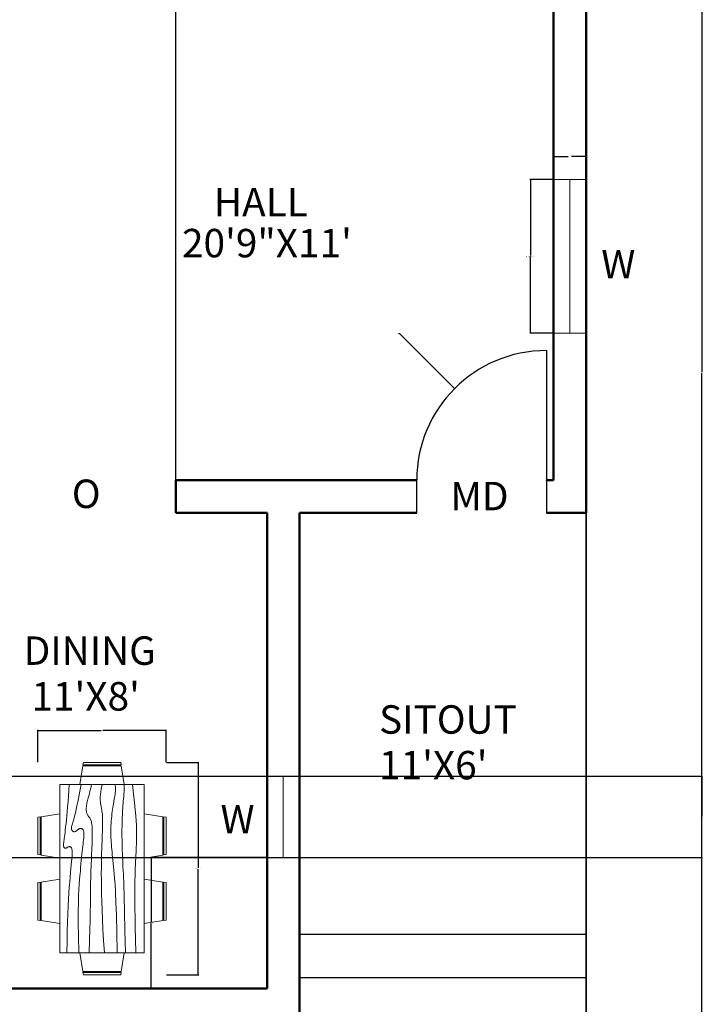
# Model space of a CAD drawing. Units: feet. Extents: x 1657 to 2001, y 1678 to 2367.
# Tile 3 of 4: x 1811 to 2001, y 1847 to 2120. Entities that reach past the tile are written whole.
import ezdxf

# ---------------------------------------------------------------- set-up
doc = ezdxf.new("R2010")
doc.units = ezdxf.units.FT
for name, color, linetype, lineweight in [('A-ANNO-DIMS', 2, 'Continuous', 18), ('A-ANNO-TEXT', 7, 'Continuous', 18), ('A-AREA-IDEN', 7, 'Continuous', 25), ('A-DOOR', 3, 'Continuous', 25), ('A-FLOR', 7, 'Continuous', 35), ('A-FLOR-STRS', 7, 'Continuous', 25), ('A-FURN', 8, 'Continuous', 18), ('A-GLAZ', 4, 'Continuous', 18), ('A-WALL', 7, 'Continuous', 50)]:
    doc.layers.add(name, color=color, linetype=linetype, lineweight=lineweight)
doc.styles.get("Standard").update_dxf_attribs({"font": 'arial.ttf'})
doc.dimstyles.get("Standard").update_dxf_attribs({"dimtxt": 0.18, "dimasz": 0.18, "dimexe": 0.18, "dimexo": 0.0625, "dimgap": 0.09, "dimtad": 0, "dimtih": 1, "dimtoh": 1, "dimdec": 4, "dimzin": 0, "dimdsep": 46, "dimtxsty": 'Standard', "dimcen": 0.09, "dimadec": 0, "dimazin": 0, "dimtfac": 1, "dimtdec": 4, "dimtofl": 0, "dimtmove": 0, "dimatfit": 3, "dimfxl": 1, "dimtolj": 1, "dimtzin": 0, "dimarcsym": 0})

# ---------------------------------------------------------------- blocks, each defined once
blk = doc.blocks.new('Dining Set - 36 x 72 in.')
for p, q in [((-22.2343, 26.00059), (-23.4847, 17.99762)), ((-22.2304, 26), (-5.7608, 26)), ((-22, 27.5), (-22.1562, 26.50042)), ((-5.8416, 26.5), (-22.1534, 26.5)), ((-22, 27.5), (-6, 27.5)), ((-5.8437, 26.49966), (-6, 27.5)), ((-4.5152, 17.99762), (-5.7655, 25.99926)), ((5.7657, 26.00059), (4.5153, 17.99762)), ((5.7696, 26), (22.2392, 26)), ((6, 27.5), (5.8438, 26.50042)), ((22.1584, 26.5), (5.8466, 26.5)), ((6, 27.5), (22, 27.5)), ((22.1563, 26.49966), (22, 27.5)), ((23.4848, 17.99762), (22.2345, 25.99926)), ((36, 18), (-36, 18)), ((-36, 18), (-36, -18)), ((36, -18), (36, 18)), ((-44.0006, 8.23428), (-35.9976, 9.48474)), ((44.0006, 8.23428), (35.9976, 9.48474)), ((-45.5, 8), (-44.5004, 8.15617)), ((-45.5, 8), (-45.5, -8)), ((-44.5, -8.15843), (-44.5, 8.15338)), ((-44, 8.23041), (-44, -8.23915)), ((44, 8.23041), (44, -8.23915)), ((44.5, -8.15843), (44.5, 8.15338)), ((45.5, 8), (44.5005, 8.15617)), ((45.5, 8), (45.5, -8)), ((-44.4997, -8.15631), (-45.5, -8)), ((-35.9976, -9.48476), (-43.9993, -8.2345)), ((35.9976, -9.48476), (43.9993, -8.2345)), ((44.4997, -8.15631), (45.5, -8)), ((-36, -18), (36, -18)), ((-22.2343, -26.0006), (-23.4847, -17.99762)), ((-4.5152, -17.99762), (-5.7655, -25.99928)), ((5.7657, -26.0006), (4.5153, -17.99762)), ((23.4848, -17.99762), (22.2345, -25.99928)), ((-22.2304, -26), (-5.7608, -26)), ((-22, -27.5), (-22.1562, -26.50044)), ((-5.8416, -26.5), (-22.1534, -26.5)), ((-22, -27.5), (-6, -27.5)), ((-5.8437, -26.49967), (-6, -27.5)), ((5.7696, -26), (22.2392, -26)), ((6, -27.5), (5.8438, -26.50044)), ((22.1584, -26.5), (5.8466, -26.5)), ((6, -27.5), (22, -27.5)), ((22.1563, -26.49967), (22, -27.5))]:
    blk.add_line(p, q)
for points in [[(-36, 15), (-31.1772, 14.97754), (-26.8079, 14.91406), (-22.8538, 14.81543), (-19.276, 14.6875), (-16.0362, 14.53613), (-13.0957, 14.36718), (-10.4159, 14.18652), (-7.9583, 14), (-5.6904, 13.81315), (-3.6035, 13.63021), (-1.6954, 13.45508), (0.0365, 13.29166), (1.5945, 13.14388), (2.9811, 13.01562), (4.1988, 12.9108), (5.25, 12.83333), (6.1393, 12.78613), (6.8802, 12.76823), (7.4883, 12.77767), (7.9792, 12.8125), (8.3685, 12.87077), (8.6719, 12.95052), (8.9049, 13.0498), (9.0833, 13.16666), (9.2205, 13.29899), (9.3216, 13.44401), (9.3895, 13.59879), (9.4271, 13.76041), (9.4373, 13.92594), (9.4232, 14.09245), (9.3875, 14.257), (9.3333, 14.41666), (9.2638, 14.56917), (9.1836, 14.71484), (9.0975, 14.85465), (9.0104, 14.98958), (8.9272, 15.1206), (8.8529, 15.2487), (8.7922, 15.37483), (8.75, 15.5), (8.7305, 15.62467), (8.7344, 15.74739), (8.7617, 15.86621), (8.8125, 15.97916), (8.8867, 16.08431), (8.9844, 16.17968), (9.1055, 16.26334), (9.25, 16.33333), (9.4189, 16.38802), (9.6172, 16.42708), (9.8506, 16.45052), (10.125, 16.45833), (10.4463, 16.45052), (10.8203, 16.42708), (11.2529, 16.38802), (11.75, 16.33333), (12.3184, 16.26318), (12.9694, 16.17838), (13.7151, 16.07991), (14.5677, 15.96875), (15.5395, 15.84586), (16.6426, 15.71224), (17.8893, 15.56884), (19.2917, 15.41666), (20.859, 15.25667), (22.5879, 15.08984), (24.4721, 14.91715), (26.5052, 14.73958), (28.6809, 14.5581), (30.9929, 14.3737), (33.4347, 14.18733), (36, 14)], [(-36, 10), (-28.9766, 10.14274), (-23.1725, 10.20442), (-18.4241, 10.19775), (-14.5677, 10.13541), (-11.4399, 10.03011), (-8.877, 9.89453), (-6.7154, 9.74137), (-4.7917, 9.58333), (-2.9698, 9.43082), (-1.2246, 9.28515), (0.4415, 9.14534), (2.026, 9.01041), (3.5266, 8.87939), (4.9408, 8.7513), (6.266, 8.62516), (7.5, 8.5), (8.6411, 8.37549), (9.6914, 8.2539), (10.6538, 8.13818), (11.5312, 8.03125), (12.3267, 7.93603), (13.043, 7.85547), (13.6831, 7.79248), (14.25, 7.75), (14.7471, 7.7303), (15.1797, 7.73307), (15.5537, 7.75732), (15.875, 7.80208), (16.1494, 7.86637), (16.3828, 7.94922), (16.5811, 8.04964), (16.75, 8.16666), (16.8944, 8.29915), (17.0143, 8.44531), (17.1089, 8.60319), (17.1771, 8.77083), (17.218, 8.94629), (17.2305, 9.1276), (17.2137, 9.31282), (17.1667, 9.5), (17.0895, 9.6875), (16.987, 9.875), (16.8649, 10.0625), (16.7292, 10.25), (16.5856, 10.4375), (16.4401, 10.625), (16.2985, 10.8125), (16.1667, 11), (16.05, 11.18733), (15.9518, 11.3737), (15.8752, 11.5581), (15.8229, 11.73958), (15.798, 11.91715), (15.8034, 12.08984), (15.842, 12.25667), (15.9167, 12.41666), (16.0295, 12.56836), (16.1784, 12.70833), (16.3605, 12.83268), (16.5729, 12.9375), (16.8127, 13.01888), (17.0768, 13.07291), (17.3625, 13.0957), (17.6667, 13.08333), (17.9894, 13.03312), (18.3418, 12.94726), (18.7382, 12.82918), (19.1927, 12.68229), (19.7195, 12.51001), (20.3327, 12.31575), (21.0465, 12.10294), (21.875, 11.875), (22.8357, 11.63354), (23.959, 11.37304), (25.2786, 11.08618), (26.8282, 10.76562), (28.6414, 10.40405), (30.752, 9.99414), (33.1936, 9.52856), (36, 9)], [(-36, 5.5), (-30.7157, 5.3348), (-26.069, 5.20963), (-21.9946, 5.11767), (-18.4271, 5.05208), (-15.3009, 5.00602), (-12.5508, 4.97265), (-10.1112, 4.94515), (-7.9167, 4.91666), (-5.909, 4.88167), (-4.0586, 4.83984), (-2.3429, 4.79215), (-0.7396, 4.73958), (0.7739, 4.6831), (2.22, 4.6237), (3.6213, 4.56233), (5, 4.5), (6.373, 4.43782), (7.7344, 4.3776), (9.0723, 4.32129), (10.375, 4.27083), (11.6309, 4.22819), (12.8281, 4.19531), (13.9551, 4.17415), (15, 4.16666), (15.954, 4.17448), (16.819, 4.19791), (17.6001, 4.23698), (18.3021, 4.29166), (18.9299, 4.36198), (19.4883, 4.44791), (19.9823, 4.54948), (20.4167, 4.66666), (20.7969, 4.79899), (21.1302, 4.94401), (21.4245, 5.09879), (21.6875, 5.26041), (21.9271, 5.42594), (22.1511, 5.59245), (22.3672, 5.757), (22.5834, 5.91666), (22.8065, 6.06868), (23.0404, 6.21093), (23.2879, 6.34147), (23.5521, 6.45833), (23.8358, 6.55957), (24.142, 6.64323), (24.4735, 6.70735), (24.8334, 6.75), (25.2235, 6.76969), (25.642, 6.76692), (26.0858, 6.74267), (26.5521, 6.69791), (27.0379, 6.63362), (27.5404, 6.55078), (28.0565, 6.45036), (28.5834, 6.33333), (29.1242, 6.19987), (29.7071, 6.04687), (30.3661, 5.87044), (31.1354, 5.66666), (32.0493, 5.43164), (33.142, 5.16146), (34.4475, 4.85221), (36, 4.5)], [(-36, -1), (-30.7915, -0.6591), (-26.0195, -0.38216), (-21.6519, -0.16284), (-17.6563, 0.00521), (-14.0005, 0.12833), (-10.6523, 0.21289), (-7.5796, 0.26522), (-4.75, 0.29166), (-2.134, 0.29793), (0.2878, 0.28711), (2.5317, 0.26163), (4.6146, 0.22396), (6.5529, 0.17651), (8.3633, 0.12174), (10.0623, 0.06209), (11.6667, 0), (13.1899, -0.06201), (14.6341, -0.1211), (15.9982, -0.17432), (17.2813, -0.21875), (18.4823, -0.25147), (19.6003, -0.26953), (20.6343, -0.27002), (21.5834, -0.25), (22.4481, -0.20768), (23.2357, -0.14584), (23.9549, -0.06836), (24.6146, 0.02083), (25.2235, 0.11784), (25.7904, 0.21875), (26.3241, 0.31966), (26.8334, 0.41666), (27.3265, 0.50618), (27.8099, 0.58593), (28.2894, 0.65397), (28.7709, 0.70833), (29.2601, 0.74707), (29.763, 0.76823), (30.2855, 0.76985), (30.8334, 0.75), (31.4088, 0.70784), (31.9994, 0.64713), (32.589, 0.57275), (33.1615, 0.48958), (33.7008, 0.4025), (34.1908, 0.3164), (34.6153, 0.23616), (34.9584, 0.16666), (35.2099, 0.11165), (35.3848, 0.07031), (35.504, 0.04069), (35.5886, 0.02083), (35.6594, 0.00879), (35.7377, 0.0026), (35.8442, 0.00032), (36, 0)], [(-36, -6.5), (-27.1843, -6.31267), (-20.084, -6.1263), (-14.469, -5.9419), (-10.1094, -5.76042), (-6.7752, -5.58285), (-4.2363, -5.41016), (-2.2629, -5.24333), (-0.625, -5.08334), (0.8708, -4.93099), (2.2715, -4.78646), (3.5872, -4.64974), (4.8281, -4.52084), (6.0046, -4.39974), (7.127, -4.28646), (8.2053, -4.18099), (9.25, -4.08334), (10.2705, -3.99382), (11.2734, -3.91407), (12.2647, -3.84603), (13.25, -3.79167), (14.2354, -3.75293), (15.2266, -3.73177), (16.2295, -3.73015), (17.25, -3.75), (18.2912, -3.79248), (19.3451, -3.85547), (20.4009, -3.93604), (21.4479, -4.03125), (22.4754, -4.13819), (23.4727, -4.25391), (24.4289, -4.37549), (25.3334, -4.5), (26.1785, -4.62492), (26.9694, -4.74935), (27.7145, -4.87281), (28.4219, -4.99479), (29.1, -5.11483), (29.7572, -5.23242), (30.4016, -5.34709), (31.0417, -5.45834), (31.6837, -5.56437), (32.3262, -5.65821), (32.9658, -5.73153), (33.599, -5.77604), (34.2224, -5.78345), (34.8327, -5.74545), (35.4264, -5.65373), (36, -5.5)], [(-36, -10), (-26.4022, -9.81299), (-18.4675, -9.62891), (-11.9839, -9.45069), (-6.7396, -9.28125), (-2.5226, -9.12354), (0.8789, -8.98047), (3.6769, -8.85498), (6.0833, -8.75), (8.2767, -8.66765), (10.3021, -8.60677), (12.1712, -8.56543), (13.8958, -8.54167), (15.4876, -8.53353), (16.9583, -8.53907), (18.3197, -8.55632), (19.5834, -8.58334), (20.7616, -8.61841), (21.8685, -8.66081), (22.9188, -8.71004), (23.9271, -8.76563), (24.9081, -8.82707), (25.8763, -8.89388), (26.8465, -8.96558), (27.8334, -9.04167), (28.8474, -9.12118), (29.8828, -9.20117), (30.93, -9.27824), (31.9792, -9.34896), (33.0205, -9.40991), (34.0443, -9.45768), (35.0407, -9.48885), (36, -9.5)], [(-36, -14.5), (-30.0881, -14.33513), (-25.0332, -14.21224), (-20.7312, -14.12647), (-17.0781, -14.07292), (-13.97, -14.04671), (-11.3027, -14.04297), (-8.9724, -14.05681), (-6.875, -14.08334), (-4.9224, -14.11833), (-3.0905, -14.16016), (-1.3709, -14.20785), (0.2448, -14.26042), (1.7647, -14.3169), (3.1973, -14.3763), (4.5507, -14.43767), (5.8333, -14.5), (7.0554, -14.5621), (8.235, -14.62175), (9.3922, -14.67652), (10.5469, -14.72396), (11.7192, -14.76164), (12.929, -14.78711), (14.1965, -14.79794), (15.5417, -14.79167), (16.9933, -14.76424), (18.6152, -14.70508), (20.4804, -14.60197), (22.6615, -14.44271), (25.2312, -14.21509), (28.2624, -13.9069), (31.8277, -13.50594), (36, -13)]]:
    blk.add_lwpolyline(points)
blk = doc.blocks.new('WIN-HALL')
for p, q in [((0, 42.59), (9, 42.59)), ((4.5, 42.59), (4.5, 0)), ((0, 0), (9, 0))]:
    blk.add_line(p, q)
blk = doc.blocks.new('*D22')
at = {"layer": 'A-ANNO-DIMS', "color": 0, "lineweight": -2, "transparency": 16777216}
for p, q in [((1851.87, 1914.01), (1860.83, 1914.01)), ((1860.65, 1913.83), (1860.65, 1884.71)), ((1860.65, 1855.22), (1860.65, 1884.34)), ((1851.87, 1855.04), (1860.83, 1855.04))]:
    blk.add_line(p, q, dxfattribs=at)
at = {"layer": 'A-ANNO-DIMS', "color": 0, "transparency": 16777216}
for points in [[(1860.62, 1913.83), (1860.68, 1913.83), (1860.65, 1914.01)], [(1860.62, 1855.22), (1860.68, 1855.22), (1860.65, 1855.04)]]:
    blk.add_solid(points, dxfattribs=at)
at = {"layer": 'Defpoints', "color": 0, "transparency": 16777216}
for p in [(1851.81, 1914.01), (1860.65, 1914.01), (1851.81, 1855.04)]:
    blk.add_point(p, dxfattribs=at)
at = {"layer": 'A-ANNO-DIMS', "color": 0, "transparency": 16777216, "insert": (1860.65, 1884.52), "char_height": 0.18, "attachment_point": 5}
blk.add_mtext('\\A1;DINING SET 59', dxfattribs=at)
blk = doc.blocks.new('*D23')
at = {"layer": 'A-ANNO-DIMS', "color": 0, "lineweight": -2, "transparency": 16777216}
for p, q in [((1816.17, 1914.07), (1816.17, 1923.03)), ((1816.35, 1922.85), (1833.77, 1922.85)), ((1851.63, 1922.85), (1834.21, 1922.85)), ((1851.81, 1914.07), (1851.81, 1923.03))]:
    blk.add_line(p, q, dxfattribs=at)
at = {"layer": 'A-ANNO-DIMS', "color": 0, "transparency": 16777216}
for points in [[(1816.35, 1922.88), (1816.35, 1922.82), (1816.17, 1922.85)], [(1851.63, 1922.88), (1851.63, 1922.82), (1851.81, 1922.85)]]:
    blk.add_solid(points, dxfattribs=at)
at = {"layer": 'Defpoints', "color": 0, "transparency": 16777216}
for p in [(1816.17, 1922.85), (1816.17, 1914.01), (1851.81, 1914.01)]:
    blk.add_point(p, dxfattribs=at)
at = {"layer": 'A-ANNO-DIMS', "color": 0, "transparency": 16777216, "insert": (1833.99, 1922.85), "char_height": 0.18, "attachment_point": 5}
blk.add_mtext('\\A1;36', dxfattribs=at)
blk = doc.blocks.new('*D30')
at = {"layer": 'A-ANNO-DIMS', "color": 0, "lineweight": -2, "transparency": 16777216}
for p, q in [((1959.22, 2075.73), (1952.72, 2075.73)), ((1952.9, 2075.55), (1952.9, 2054.62)), ((1952.9, 2033.32), (1952.9, 2054.25)), ((1959.22, 2033.14), (1952.72, 2033.14))]:
    blk.add_line(p, q, dxfattribs=at)
at = {"layer": 'A-ANNO-DIMS', "color": 0, "transparency": 16777216}
for points in [[(1952.87, 2075.55), (1952.93, 2075.55), (1952.9, 2075.73)], [(1952.87, 2033.32), (1952.93, 2033.32), (1952.9, 2033.14)]]:
    blk.add_solid(points, dxfattribs=at)
at = {"layer": 'Defpoints', "color": 0, "transparency": 16777216}
for p in [(1959.28, 2075.73), (1952.9, 2033.14), (1959.28, 2033.14)]:
    blk.add_point(p, dxfattribs=at)
at = {"layer": 'A-ANNO-DIMS', "color": 0, "transparency": 16777216, "insert": (1952.9, 2054.44), "char_height": 0.18, "attachment_point": 5}
blk.add_mtext('\\A1;HALL WINDOW 43 TYP.', dxfattribs=at)
blk = doc.blocks.new('*D31')
at = {"layer": 'A-ANNO-DIMS', "color": 0, "lineweight": -2, "transparency": 16777216}
for p, q in [((1959.28, 2075.79), (1959.28, 2082.3)), ((1959.46, 2082.12), (1963.33, 2082.12)), ((1968.1, 2082.12), (1964.24, 2082.12)), ((1968.28, 2075.79), (1968.28, 2082.3))]:
    blk.add_line(p, q, dxfattribs=at)
at = {"layer": 'A-ANNO-DIMS', "color": 0, "transparency": 16777216}
for points in [[(1959.46, 2082.15), (1959.46, 2082.09), (1959.28, 2082.12)], [(1968.1, 2082.15), (1968.1, 2082.09), (1968.28, 2082.12)]]:
    blk.add_solid(points, dxfattribs=at)
at = {"layer": 'Defpoints', "color": 0, "transparency": 16777216}
for p in [(1959.28, 2082.12), (1959.28, 2075.73), (1968.28, 2075.73)]:
    blk.add_point(p, dxfattribs=at)
at = {"layer": 'A-ANNO-DIMS', "color": 0, "transparency": 16777216, "insert": (1963.78, 2082.12), "char_height": 0.18, "attachment_point": 5}
blk.add_mtext('\\A1;9 TYP.', dxfattribs=at)
blk = doc.blocks.new('*D35')
at = {"layer": 'A-ANNO-DIMS', "color": 0, "lineweight": -2, "transparency": 16777216}
for p, q in [((1968.35, 2334.3), (2000.61, 2334.3)), ((2000.43, 2334.12), (2000.43, 2022.48)), ((2000.43, 1710.48), (2000.43, 2022.12)), ((1968.35, 1710.3), (2000.61, 1710.3))]:
    blk.add_line(p, q, dxfattribs=at)
at = {"layer": 'A-ANNO-DIMS', "color": 0, "transparency": 16777216}
for points in [[(2000.4, 2334.12), (2000.46, 2334.12), (2000.43, 2334.3)], [(2000.4, 1710.48), (2000.46, 1710.48), (2000.43, 1710.3)]]:
    blk.add_solid(points, dxfattribs=at)
at = {"layer": 'Defpoints', "color": 0, "transparency": 16777216}
for p in [(1968.28, 2334.3), (2000.43, 2334.3), (1968.28, 1710.3)]:
    blk.add_point(p, dxfattribs=at)
at = {"layer": 'A-ANNO-DIMS', "color": 0, "transparency": 16777216, "insert": (2000.43, 2022.3), "char_height": 0.18, "attachment_point": 5}
blk.add_mtext('\\A1;624', dxfattribs=at)
blk = doc.blocks.new('*D54')
at = {"layer": 'A-ANNO-DIMS', "color": 0, "lineweight": -2, "transparency": 16777216}
for p, q in [((1779.35, 1910.16), (2000.61, 1910.16)), ((2000.43, 1909.98), (2000.43, 1899.06)), ((2000.43, 1887.77), (2000.43, 1898.69)), ((1779.35, 1887.59), (2000.61, 1887.59))]:
    blk.add_line(p, q, dxfattribs=at)
at = {"layer": 'A-ANNO-DIMS', "color": 0, "transparency": 16777216}
for points in [[(2000.4, 1909.98), (2000.46, 1909.98), (2000.43, 1910.16)], [(2000.4, 1887.77), (2000.46, 1887.77), (2000.43, 1887.59)]]:
    blk.add_solid(points, dxfattribs=at)
at = {"layer": 'Defpoints', "color": 0, "transparency": 16777216}
for p in [(1779.28, 1910.16), (2000.43, 1910.16), (1779.28, 1887.59)]:
    blk.add_point(p, dxfattribs=at)
at = {"layer": 'A-ANNO-DIMS', "color": 0, "transparency": 16777216, "insert": (2000.43, 1898.88), "char_height": 0.18, "attachment_point": 5}
blk.add_mtext('\\A1;22.577', dxfattribs=at)
blk = doc.blocks.new('*D56')
at = {"layer": 'A-ANNO-DIMS', "color": 0, "lineweight": -2, "transparency": 16777216}
for p, q in [((1802.91, 1992.36), (1802.91, 2366.63)), ((1803.09, 2366.45), (1828.29, 2366.45)), ((1854.28, 2366.45), (1829.08, 2366.45)), ((1854.46, 1992.36), (1854.46, 2366.63))]:
    blk.add_line(p, q, dxfattribs=at)
at = {"layer": 'A-ANNO-DIMS', "color": 0, "transparency": 16777216}
for points in [[(1803.09, 2366.48), (1803.09, 2366.42), (1802.91, 2366.45)], [(1854.28, 2366.48), (1854.28, 2366.42), (1854.46, 2366.45)]]:
    blk.add_solid(points, dxfattribs=at)
at = {"layer": 'Defpoints', "color": 0, "transparency": 16777216}
for p in [(1854.46, 2366.45), (1802.91, 1992.3), (1854.46, 1992.3)]:
    blk.add_point(p, dxfattribs=at)
at = {"layer": 'A-ANNO-DIMS', "color": 0, "transparency": 16777216, "insert": (1828.68, 2366.45), "char_height": 0.18, "attachment_point": 5}
blk.add_mtext('\\A1;51.55', dxfattribs=at)
blk = doc.blocks.new('*D57')
at = {"layer": 'A-ANNO-DIMS', "color": 0, "lineweight": -2, "transparency": 16777216}
for p, q in [((1879.72, 1887.59), (1847.45, 1887.59)), ((1847.63, 1887.41), (1847.63, 1869.62)), ((1847.63, 1851.48), (1847.63, 1869.26)), ((1879.72, 1851.3), (1847.45, 1851.3))]:
    blk.add_line(p, q, dxfattribs=at)
at = {"layer": 'A-ANNO-DIMS', "color": 0, "transparency": 16777216}
for points in [[(1847.6, 1887.41), (1847.66, 1887.41), (1847.63, 1887.59)], [(1847.6, 1851.48), (1847.66, 1851.48), (1847.63, 1851.3)]]:
    blk.add_solid(points, dxfattribs=at)
at = {"layer": 'Defpoints', "color": 0, "transparency": 16777216}
for p in [(1847.63, 1887.59), (1879.78, 1887.59), (1879.78, 1851.3)]:
    blk.add_point(p, dxfattribs=at)
at = {"layer": 'A-ANNO-DIMS', "color": 0, "transparency": 16777216, "insert": (1847.63, 1869.44), "char_height": 0.18, "attachment_point": 5}
blk.add_mtext('\\A1;36.29', dxfattribs=at)
blk = doc.blocks.new('*D58')
at = {"layer": 'A-ANNO-DIMS', "color": 0, "lineweight": -2, "transparency": 16777216}
for p, q in [((1888.85, 1910.16), (2000.61, 1910.16)), ((2000.43, 1909.98), (2000.43, 1899.06)), ((2000.43, 1887.77), (2000.43, 1898.69)), ((1888.85, 1887.59), (2000.61, 1887.59))]:
    blk.add_line(p, q, dxfattribs=at)
at = {"layer": 'A-ANNO-DIMS', "color": 0, "transparency": 16777216}
for points in [[(2000.4, 1909.98), (2000.46, 1909.98), (2000.43, 1910.16)], [(2000.4, 1887.77), (2000.46, 1887.77), (2000.43, 1887.59)]]:
    blk.add_solid(points, dxfattribs=at)
at = {"layer": 'Defpoints', "color": 0, "transparency": 16777216}
for p in [(1888.78, 1910.16), (2000.43, 1910.16), (1888.78, 1887.59)]:
    blk.add_point(p, dxfattribs=at)
at = {"layer": 'A-ANNO-DIMS', "color": 0, "transparency": 16777216, "insert": (2000.43, 1898.88), "char_height": 0.18, "attachment_point": 5}
blk.add_mtext('\\A1;22.577', dxfattribs=at)
blk = doc.blocks.new('*D59')
at = {"layer": 'A-ANNO-DIMS', "color": 0, "lineweight": -2, "transparency": 16777216}
for p, q in [((1916.38, 2033.03), (1916.56, 2033.03)), ((1916.56, 2033.03), (1931.7, 2017.88)), ((1957.19, 1992.3), (1957.37, 1992.3)), ((1957.28, 1992.21), (1957.28, 1992.39))]:
    blk.add_line(p, q, dxfattribs=at)
at = {"layer": 'A-ANNO-DIMS', "color": 0, "transparency": 16777216}
blk.add_solid([(1931.72, 2017.9), (1931.68, 2017.86), (1931.83, 2017.75)], dxfattribs=at)
at = {"layer": 'Defpoints', "color": 0, "transparency": 16777216}
for p in [(1931.83, 2017.75), (1957.28, 1992.3)]:
    blk.add_point(p, dxfattribs=at)
at = {"layer": 'A-ANNO-DIMS', "color": 0, "transparency": 16777216, "insert": (1916.07, 2033.03), "char_height": 0.18, "attachment_point": 5}
blk.add_mtext('\\A1;R36', dxfattribs=at)

msp = doc.modelspace()

# ---------------------------------------------------------------- linework, layer by layer
at = {"layer": 'A-DOOR'}
for p, q in [((1957.2848, 2028.2977), (1957.2848, 1983.2977)), ((1921.2848, 1983.2977), (1921.2848, 1992.2977))]:
    msp.add_line(p, q, dxfattribs=at)
msp.add_arc((1957.2848, 1992.2977), 36, 90, 180, dxfattribs=at)
at = {"layer": 'A-FLOR'}
msp.add_line((1968.2848, 1842.2977), (1968.2848, 1983.2977), dxfattribs=at)
at = {"layer": 'A-FLOR-STRS'}
for p, q in [((1888.7848, 1866.2977), (1968.2848, 1866.2977)), ((1888.7848, 1854.2977), (1968.2848, 1854.2977))]:
    msp.add_line(p, q, dxfattribs=at)
at = {"layer": 'A-GLAZ'}
for p, q in [((1879.7848, 1910.1638), (1888.7848, 1910.1638)), ((1884.2848, 1910.1638), (1884.2848, 1887.5865)), ((1879.7848, 1887.5865), (1888.7848, 1887.5865))]:
    msp.add_line(p, q, dxfattribs=at)
at = {"layer": 'A-WALL'}
for p, q in [((1968.2848, 2334.2977), (1968.2848, 1983.2977)), ((1959.2848, 2123.2751), (1959.2848, 1992.2977)), ((1854.4579, 1992.2977), (1854.4579, 1983.2977)), ((1854.4579, 1992.2977), (1921.2848, 1992.2977)), ((1957.2848, 1992.2977), (1959.2848, 1992.2977)), ((1854.4579, 1983.2977), (1879.7848, 1983.2977)), ((1879.7848, 1851.2977), (1879.7848, 1983.2977)), ((1888.7848, 1851.2977), (1888.7848, 1983.2977)), ((1888.7848, 1983.2977), (1921.2848, 1983.2977)), ((1957.2848, 1983.2977), (1968.2848, 1983.2977)), ((1783.7848, 1851.2977), (1879.7848, 1851.2977)), ((1888.7848, 1851.2977), (1888.7848, 1842.2977))]:
    msp.add_line(p, q, dxfattribs=at)

# ---------------------------------------------------------------- block references
at = {"layer": 'A-FURN', "xscale": 0.647979979263925, "yscale": 0.647979979263925, "zscale": 0.647979979263925, "rotation": 90}
msp.add_blockref('Dining Set - 36 x 72 in.', (1833.9897, 1884.5221), dxfattribs=at)
at = {"layer": 'A-GLAZ', "rotation": 180}
msp.add_blockref('WIN-HALL', (1968.2845, 2075.7291), dxfattribs=at)

# ---------------------------------------------------------------- texts
at = {"layer": 'A-ANNO-TEXT'}
for s, height, p in [('W', 7.8904, (1972.4989, 2048.2939)), ('O', 7.8904, (1825.6131, 1984.5938)), ('MD', 7.89038, (1930.6333, 1983.9585)), ('W', 7.8904, (1866.8571, 1894.2918))]:
    msp.add_text(s, height=height, dxfattribs=at).set_placement(p)
at = {"layer": 'A-AREA-IDEN'}
for s, p in [('HALL', (1865.0159, 2065.4942)), ('20\'9"X11\'', (1856.173, 2054.1554)), ('DINING', (1812.2415, 1941.072)), ("11'X8'", (1814.4163, 1928.3968)), ('SITOUT', (1910.8545, 1921.9636)), ("11'X6'", (1910.8545, 1909.2884))]:
    msp.add_text(s, height=7.89038, dxfattribs=at).set_placement(p)

# ---------------------------------------------------------------- dimensions: what is measured, and where the dimension line sits
at = {"layer": 'A-ANNO-DIMS'}
dim = msp.add_linear_dim(base=(1854.4579, 2366.4477), p1=(1802.9077, 1992.2977), p2=(1854.4579, 1992.2977), dimstyle='Standard', override={"dimdec": 2, "dimlfac": 1, "dimrnd": 0, "dimzin": 0, "dimdsep": 46, "dimlunit": 2}, dxfattribs=at)
dim.commit()
dim.dimension.update_dxf_attribs({"geometry": '*D56', "text_midpoint": (1828.6828, 2366.4477)})
for base, p1, p2, angle, override, picture, middle in [((2000.4348, 2334.2977), (1968.2848, 1710.2977), (1968.2848, 2334.2977), 90, {"dimdec": 0, "dimlfac": 1, "dimrnd": 0, "dimzin": 0, "dimdsep": 46, "dimlunit": 2}, '*D35', (2000.4348, 2022.2977)), ((1816.1703, 1922.8501), (1851.8092, 1914.0051), (1816.1703, 1914.0051), 180, {"dimdec": 0, "dimlfac": 1, "dimrnd": 0, "dimzin": 0, "dimdsep": 46, "dimlunit": 2}, '*D23', (1833.9897, 1922.8501)), ((2000.4348, 1910.1638), (1779.2848, 1887.5865), (1779.2848, 1910.1638), 90, {"dimdec": 3, "dimlfac": 1, "dimrnd": 0, "dimzin": 0, "dimdsep": 46, "dimlunit": 2}, '*D54', (2000.4348, 1898.8751)), ((2000.4348, 1910.1638), (1888.7848, 1887.5865), (1888.7848, 1910.1638), 90, {"dimdec": 3, "dimlfac": 1, "dimrnd": 0, "dimzin": 0, "dimdsep": 46, "dimlunit": 2}, '*D58', (2000.4348, 1898.8751)), ((1847.6348, 1887.5865), (1879.7848, 1851.2977), (1879.7848, 1887.5865), 90, {"dimdec": 2, "dimlfac": 1, "dimrnd": 0, "dimzin": 0, "dimdsep": 46, "dimlunit": 2}, '*D57', (1847.6348, 1869.4421))]:
    dim = msp.add_linear_dim(base=base, p1=p1, p2=p2, angle=angle, dimstyle='Standard', override=override, dxfattribs=at)
    dim.commit()
    dim.dimension.update_dxf_attribs({"geometry": picture, "text_midpoint": middle})
for base, p1, p2, angle, text, picture, middle in [((1959.2848, 2082.1168), (1968.2848, 2075.729), (1959.2848, 2075.729), 180, '<> TYP.', '*D31', (1963.7848, 2082.1168)), ((1952.897, 2033.144), (1959.2848, 2075.729), (1959.2848, 2033.144), 270, 'HALL WINDOW <> TYP.', '*D30', (1952.897, 2054.4365)), ((1860.6541, 1914.0051), (1851.8092, 1855.039), (1851.8092, 1914.0051), 90, 'DINING SET <>', '*D22', (1860.6541, 1884.5221))]:
    dim = msp.add_linear_dim(base=base, p1=p1, p2=p2, angle=angle, text=text, dimstyle='Standard', override={"dimdec": 0, "dimlfac": 1, "dimrnd": 0, "dimzin": 0, "dimdsep": 46, "dimlunit": 2}, dxfattribs=at)
    dim.commit()
    dim.dimension.update_dxf_attribs({"geometry": picture, "text_midpoint": middle})
dim = msp.add_radius_dim(center=(1957.2848, 1992.2977), mpoint=(1931.8292, 2017.7538), dimstyle='Standard', override={"dimdec": 0, "dimlfac": 1, "dimrnd": 0, "dimzin": 0, "dimdsep": 46, "dimlunit": 2}, dxfattribs=at)
dim.commit()
dim.dimension.update_dxf_attribs({"geometry": '*D59', "text_midpoint": (1916.0709, 2033.0275), "dimtype": 164})

doc.saveas('drawing.dxf')
